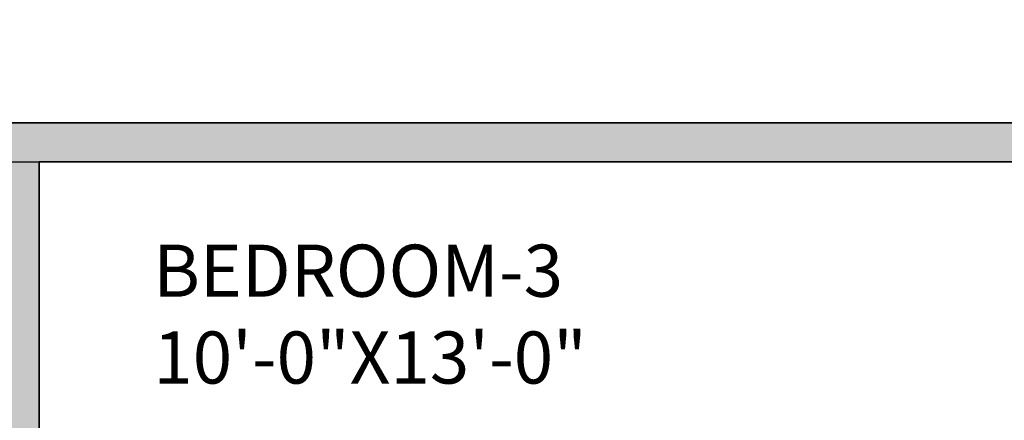
# Model space of a CAD drawing. Units: inches. Extents: x -15 to 423, y -713 to 71.
# Tile 16 of 24: x 251 to 364, y -270 to -224. Entities that reach past the tile are written whole.
import ezdxf

# ---------------------------------------------------------------- set-up
doc = ezdxf.new("R2010")
doc.units = ezdxf.units.IN
doc.header["$MEASUREMENT"] = 0
for name, color, linetype, lineweight in [('A-ANNO-DIMS', 2, 'Continuous', 18), ('A-AREA-IDEN', 7, 'Continuous', 18), ('A-WALL', 7, 'Continuous', 35), ('A-WALL-PATT', 8, 'Continuous', 13)]:
    doc.layers.add(name, color=color, linetype=linetype, lineweight=lineweight)
doc.styles.get("Standard").update_dxf_attribs({"font": 'arial.ttf'})
doc.dimstyles.get("Standard").update_dxf_attribs({"dimtxt": 0.18, "dimasz": 0.18, "dimexe": 0.18, "dimexo": 0.0625, "dimgap": 0.09, "dimtad": 0, "dimtih": 1, "dimtoh": 1, "dimdec": 0, "dimzin": 0, "dimdsep": 46, "dimlunit": 3, "dimtxsty": 'Standard', "dimcen": 0.09, "dimadec": 0, "dimazin": 0, "dimtfac": 1, "dimtdec": 0, "dimtofl": 0, "dimtmove": 0, "dimatfit": 3, "dimfxl": 1, "dimtolj": 1, "dimtzin": 0, "dimarcsym": 0})

# ---------------------------------------------------------------- blocks, each defined once
blk = doc.blocks.new('*D38')
at = {"layer": 'A-ANNO-DIMS', "color": 0, "lineweight": -2, "transparency": 16777216}
for p, q in [((124.14, -240.5), (422.01, -240.5)), ((421.83, -240.68), (421.83, -258.06)), ((421.83, -275.8), (421.83, -258.42)), ((124.14, -275.98), (422.01, -275.98))]:
    blk.add_line(p, q, dxfattribs=at)
at = {"layer": 'A-ANNO-DIMS', "color": 0, "transparency": 16777216}
for points in [[(421.8, -240.68), (421.86, -240.68), (421.83, -240.5)], [(421.8, -275.8), (421.86, -275.8), (421.83, -275.98)]]:
    blk.add_solid(points, dxfattribs=at)
at = {"layer": 'Defpoints', "color": 0, "transparency": 16777216}
for p in [(124.08, -240.5), (124.08, -275.98), (421.83, -275.98)]:
    blk.add_point(p, dxfattribs=at)
at = {"layer": 'A-ANNO-DIMS', "color": 0, "transparency": 16777216, "insert": (421.83, -258.24), "char_height": 0.18, "attachment_point": 5}
blk.add_mtext('\\A1;2\'-11 1/2"', dxfattribs=at)

msp = doc.modelspace()

# ---------------------------------------------------------------- hatches: boundary and pattern name
at = {"layer": 'A-WALL-PATT'}
h = msp.add_hatch(color=256, dxfattribs=at)
h.dxf.hatch_style = 1
h.paths.add_polyline_path([(34.08, -349.58), (25.08, -349.58), (25.08, -431), (34.08, -431)])
h.paths.add_polyline_path([(34.08, -467), (25.08, -467), (25.08, -673), (34.08, -673)])
h.paths.add_polyline_path([(373.08, -668.5), (182.08, -668.5), (182.08, -673), (373.08, -673)])
h.paths.add_polyline_path([(253.2, -597.5), (191.08, -597.5), (191.08, -594.5), (182.08, -594.5), (182.08, -606.5), (253.2, -606.5)])
h.paths.add_polyline_path([(373.08, -597.5), (313.2, -597.5), (313.2, -606.5), (373.08, -606.5)])
h.paths.add_polyline_path([(382.08, -545.55), (373.08, -545.55), (373.08, -673), (382.08, -673)])
h.paths.add_polyline_path([(139.08, -488), (34.08, -488), (34.08, -497), (139.08, -497), (139.08, -492.5)])
h.paths.add_polyline_path([(139.08, -396.5), (128.58, -396.5), (128.58, -352.79), (124.08, -352.79), (124.08, -396.5), (34.08, -396.5), (34.08, -410), (139.08, -410), (139.08, -403.25)])
h.paths.add_polyline_path([(191.08, -396.5), (179.08, -396.5), (179.08, -410), (182.08, -410), (182.08, -488), (179.08, -488), (179.08, -497), (182.08, -497), (182.08, -501.43), (191.08, -501.43)])
h.paths.add_polyline_path([(373.08, -396.5), (253.08, -396.5), (253.08, -393.5), (248.58, -393.5), (248.58, -401), (284.58, -401), (284.58, -404), (289.08, -404), (289.08, -401), (373.08, -401)])
h.paths.add_polyline_path([(373.08, -449), (289.08, -449), (289.08, -432), (286.83, -432), (284.58, -432), (284.58, -453.5), (373.08, -453.5)])
h.paths.add_polyline_path([(382.08, -344.27), (373.08, -344.27), (373.08, -413.68), (382.08, -413.68)])
h.paths.add_polyline_path([(382.08, -437.68), (373.08, -437.68), (373.08, -485.55), (382.08, -485.55)])
h.paths.add_polyline_path([(34.08, -188.26), (25.08, -188.26), (25.08, -289.58), (34.08, -289.58)])
h.paths.add_polyline_path([(164.08, -236), (34.08, -236), (34.08, -240.5), (124.08, -240.5), (124.08, -293.12), (128.58, -293.12), (128.58, -240.5), (164.08, -240.5), (164.08, -238.25)])
h.paths.add_polyline_path([(373.08, -236), (242.58, -236), (242.58, -238.25), (242.58, -240.5), (248.58, -240.5), (248.58, -353.5), (250.83, -353.5), (253.08, -353.5), (253.08, -240.5), (373.08, -240.5)])
h.paths.add_polyline_path([(382.08, -190.86), (373.08, -190.86), (373.08, -284.27), (382.08, -284.27)])
h.paths.add_polyline_path([(211.58, -80), (253.58, -80), (253.58, -77.75), (253.58, -75.5), (153.58, -75.5), (153.58, -77.75), (153.58, -80), (207.08, -80), (207.08, -236), (204.08, -236), (204.08, -240.5), (214.58, -240.5), (214.58, -236), (211.58, -236)])
h.paths.add_polyline_path([(34.08, 8.5), (70.36, 8.5), (70.36, 17.5), (25.08, 17.5), (25.08, -128.26), (34.08, -128.26)])
h.paths.add_polyline_path([(110.58, 17.5), (94.36, 17.5), (94.36, 8.5), (110.58, 8.5)])
h.paths.add_polyline_path([(296.58, 17.5), (110.58, 17.5), (110.58, 13), (296.58, 13)])
h.paths.add_polyline_path([(110.58, 8.5), (106.08, 8.5), (106.08, -75.5), (103.08, -75.5), (103.08, -80), (113.58, -80), (113.58, -77.75), (113.58, -75.5), (110.58, -75.5)])
h.paths.add_polyline_path([(75.08, -75.5), (34.08, -75.5), (34.08, -80), (75.08, -80), (75.08, -77.75)])
h.paths.add_polyline_path([(343.09, 17.5), (296.58, 17.5), (296.58, 13), (296.58, 8.5), (343.09, 8.5)])
h.paths.add_polyline_path([(304.08, -75.5), (301.08, -75.5), (301.08, 8.5), (296.58, 8.5), (296.58, -75.5), (293.58, -75.5), (293.58, -80), (304.08, -80)])
h.paths.add_polyline_path([(382.08, 17.5), (367.09, 17.5), (367.09, 8.5), (373.08, 8.5), (373.08, -130.86), (382.08, -130.86)])
h.paths.add_polyline_path([(373.08, -75.5), (332.08, -75.5), (332.08, -77.75), (332.08, -80), (373.08, -80)])

# ---------------------------------------------------------------- linework, layer by layer
at = {"layer": 'A-WALL'}
for p, q in [((242.58, -236), (373.08, -236)), ((253.08, -240.5), (253.08, -353.5)), ((253.08, -240.5), (373.08, -240.5))]:
    msp.add_line(p, q, dxfattribs=at)

# ---------------------------------------------------------------- texts
at = {"layer": 'A-AREA-IDEN', "insert": (266.22, -250.03), "char_height": 6, "attachment_point": 1}
msp.add_mtext('BEDROOM-3\\P10\'-0"X13\'-0"', dxfattribs=at)

# ---------------------------------------------------------------- dimensions: what is measured, and where the dimension line sits
at = {"layer": 'A-ANNO-DIMS'}
dim = msp.add_linear_dim(base=(421.83, -275.98), p1=(124.08, -240.5), p2=(124.08, -275.98), angle=90, dimstyle='Standard', override={"dimdec": 1, "dimlfac": 1, "dimrnd": 0, "dimzin": 1, "dimdsep": 46, "dimlunit": 4, "dimfrac": 2}, dxfattribs=at)
dim.commit()
dim.dimension.update_dxf_attribs({"geometry": '*D38', "text_midpoint": (421.83, -258.24)})

doc.saveas('drawing.dxf')
